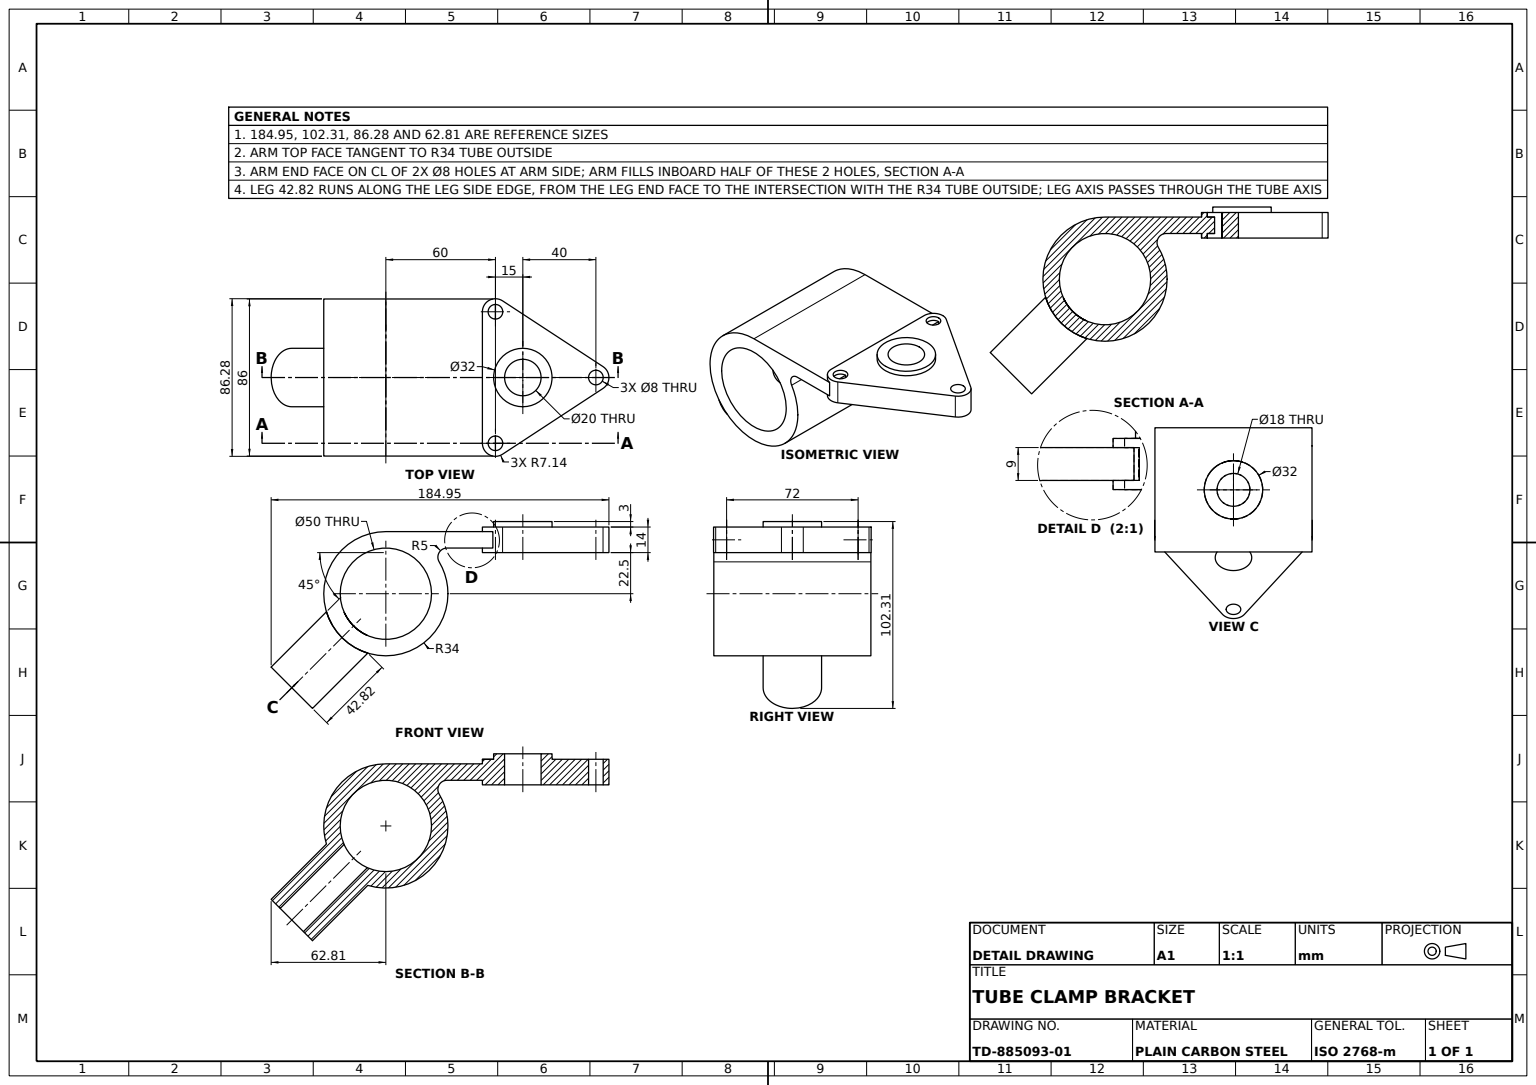
SolidWorks part; units mm, degrees
material "Plain Carbon Steel"
ref_plane "Front Plane" through (0, 0, 0) normal (0, 0, 1) x (1, 0, 0)
ref_plane "Top Plane" through (0, 0, 0) normal (0, 1, 0) x (1, 0, 0)
ref_plane "Right Plane" through (0, 0, 0) normal (1, 0, 0) x (0, 0, -1)
sketch "Ring Hub Profile" plane through (0, 0, 0) normal (0, 0, 1) x (1, 0, 0)
  line L0 (0, 34) -> (60, 34)
  line L1 (33.4813, 25) -> (60, 25)
  line L2 (60, 34) -> (60, 25)
  line L3 (0, 25) -> (60, 25) construction
  circle A0 centre (0, 0) radius 25
  arc A1 (0, 34) -> (29.1889, 17.4359) centre (0, 0) ccw
  arc A2 (33.4813, 25) -> (29.1889, 17.4359) centre (33.4813, 20) ccw
  dimension "D1" = 68
  dimension "D2" = 50
  dimension "D4" = 5
  dimension "D5" = 60
  dimension "D3" = 9
extrude "Ring Hub" add sketch "Ring Hub Profile" along normal mid plane 86
ref_plane "Flange Plane" through (0, 29.5, 0) normal (0, 1, 0) x (1, 0, 0)
sketch "Flange Profile 3 Holes" plane through (0, 29.5, 0) normal (0, 1, 0) x (1, 0, 0)
  line L7 (63.9109, 41.9751) -> (118.9109, 5.9751)
  line L8 (63.9109, -41.9751) -> (118.9109, -5.9751)
  line L9 (52.8588, 36) -> (52.8588, -36)
  circle A0 centre (60, 36) radius 4
  circle A1 centre (60, -36) radius 4
  circle A2 centre (75, 0) radius 25.9717 construction
  circle A3 centre (115, 0) radius 4
  arc A4 (52.8588, -36) -> (63.9109, -41.9751) centre (60, -36) ccw
  arc A5 (63.9109, 41.9751) -> (52.8588, 36) centre (60, 36) ccw
  arc A6 (118.9109, -5.9751) -> (118.9109, 5.9751) centre (115, 0) ccw
  dimension "D3" = 8
  dimension "D4" = 8
  dimension "D7" = 8
  dimension "D9" = 14.2824
  dimension "D10" = 51.9433
  dimension "D1" = 72
  dimension "D2" = 36
  dimension "D5" = 15
  dimension "D6" = 75
  dimension "D8" = 40
extrude "Triangular Flange" add sketch "Flange Profile 3 Holes" along normal mid plane 14
sketch "Flange Boss Profile" plane through (0, 36.5, 0) normal (0, 1, 0) x (1, 0, 0)
  line L0 (115, 0) -> (-53.4073, 0) construction
  line L1 (58.5869, -43) -> (0, -43) construction
  circle A0 centre (75, 0) radius 16
  circle A1 centre (75, 0) radius 10
  dimension "D1" = 32
  dimension "D2" = 20
  dimension "D3" = 75
  dimension "D4" = 43
sketch "Boss Bore Profile" plane through (0, 29.5, 0) normal (0, 1, 0) x (1, 0, 0)
  circle A1 centre (75, 0) radius 10
  circle A2 centre (75, 0) radius 10
  dimension "D1" = 0
extrude "Boss Bore" cut sketch "Boss Bore Profile" against normal mid plane 26
extrude "Flange Boss Ø32" add sketch "Flange Boss Profile" along normal blind 3
sketch "Hub Revolve Profile" plane through (0, 0, 0) normal (0, 0, 1) x (1, 0, 0)
  line L1 (0, 0) -> (-51.4914, -51.4914) construction
  line L2 (-32.5269, -9.8995) -> (-62.8051, -40.1777)
  line L4 (-62.8051, -40.1777) -> (-57.8553, -45.1274)
  line L5 (-57.8553, -45.1274) -> (-29.548, -16.8201)
  line L7 (-34, 0) -> (-57.6921, 0) construction
  line L8 (-11.3137, 11.3137) -> (-62.8051, -40.1777) construction
  arc A0 (0, 34) -> (29.1889, 17.4359) centre (0, 0) ccw construction
  arc A1 (-32.5269, -9.8995) -> (-29.548, -16.8201) centre (0, 0) ccw
  dimension "D1" = 4.9497
  dimension "D4" = 9
  dimension "D5" = 9.8995
  dimension "D3" = 30.2782
  dimension "D2" = 16
revolve "Hub Revolved Feature" add sketch "Hub Revolve Profile" angle 360 about L1
sketch "Hub Slit Profile" plane through (-51.4914, -51.4914, 0) normal (-0.7071, -0.7071, 0) x (0, 0, 1)
  circle A0 centre (0, 0) radius 9 construction
  circle A1 centre (0, 0) radius 9
extrude "Hub Slit Cut" cut sketch "Hub Slit Profile" against normal mid plane 135
